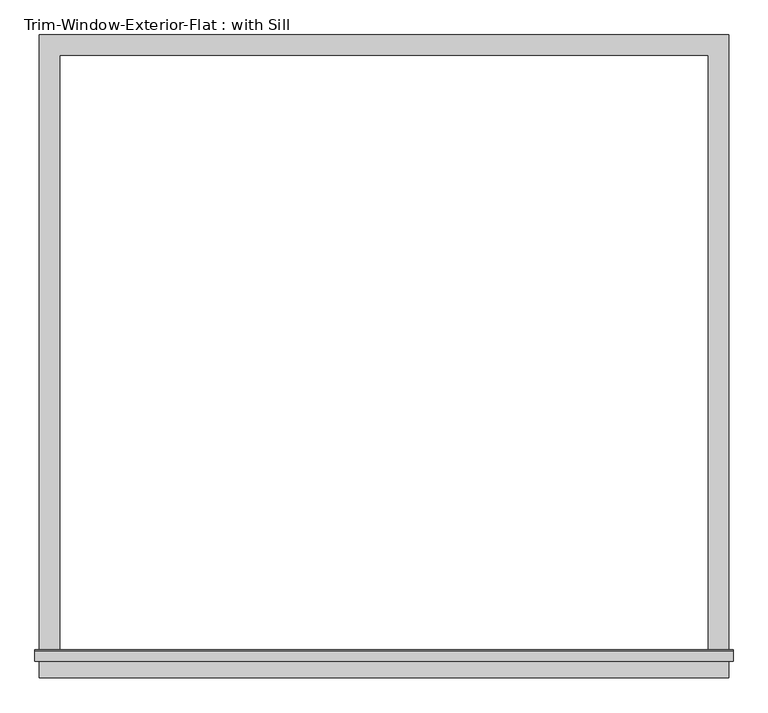
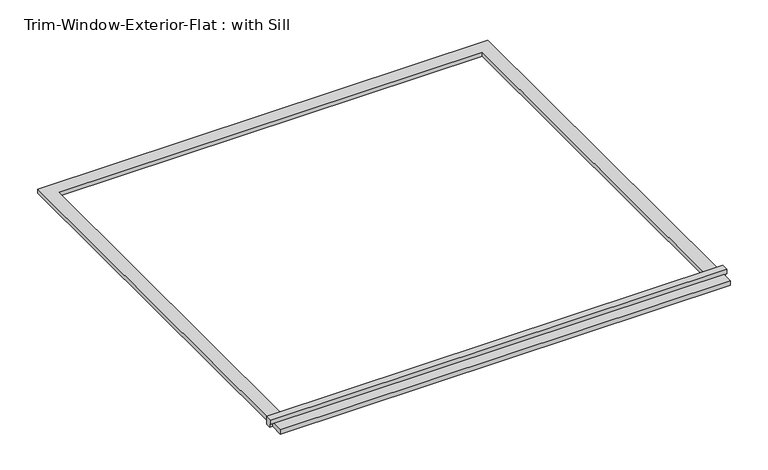
"""IFC4 building model written with IfcOpenShell, lengths in millimetres: proxy geometry, Trim-Window-Exterior-Flat : with Sill."""

from ifc_helpers import new_model, si_unit, frame, origin, origin_with_axes, place, context, project, spatial, polyline, outline, extrude, source, transform, mapped, element, save


def trim_window_exterior_flat_with_sill_c98b2dec(model_context):
    return source(origin(), model_context, "Body", "SweptSolid", [
        extrude(outline(polyline([(971.55, -1698.5823709), (971.55, -1755.7323709), (-971.55, -1755.7323709), (-971.55, -1698.5823709), (971.55, -1698.5823709)])), origin_with_axes(), (0.0, 0.0, 1.0), 19.05),
        extrude(outline(polyline([(-1708.15, 38.1), (-1678.8580645, 38.1), (-1676.4, 19.05), (-1676.4, 0.0), (-1698.5823709, 0.0), (-1698.5823709, 19.05), (-1708.15, 19.05), (-1708.15, 38.1)])), frame((-984.25, 0.0, 0.0), z_axis=(1.0, 0.0, 0.0), x_axis=(0.0, 1.0, 0.0)), (0.0, 0.0, 1.0), 1968.5),
        extrude(outline(polyline([(-971.55, 57.15), (971.55, 57.15), (971.55, -1676.4), (914.4, -1676.4), (914.4, 0.0), (-914.4, 0.0), (-914.4, -1676.4), (-971.55, -1676.4), (-971.55, 57.15)])), origin_with_axes(), (0.0, 0.0, 1.0), 19.05),
    ])


if __name__ == "__main__":
    model = new_model("IFC4")
    model_context = context("Model", 3, world=origin())
    ifc_project = project(units=[si_unit("LENGTHUNIT", "METRE", prefix="MILLI")], contexts=[model_context])
    site = spatial("IfcSite", under=ifc_project)
    building = spatial("IfcBuilding", under=site)
    placement = place(None, origin())
    trim_window_exterior_flat_with_sill_shape = trim_window_exterior_flat_with_sill_c98b2dec(model_context)
    element("IfcBuildingElementProxy", 1, Name="Trim-Window-Exterior-Flat : with Sill", ObjectType="Trim-Window-Exterior-Flat : with Sill", at=placement, inside=building, context=model_context, shape_type="MappedRepresentation", body=[
        mapped(trim_window_exterior_flat_with_sill_shape, transform((0.0, 0.0, 0.0), x_axis=(1.0, 0.0, 0.0), y_axis=(0.0, 1.0, 0.0), z_axis=(0.0, 0.0, 1.0))),
    ])
    save(model, "model.ifc")

# Revit data of these elements
# Type "Trim-Window-Exterior-Flat : with Sill"
#   Trim Width = 0' - 2 1/4"
#   Trim Thickness_Picture Frame = 0' - 1 1/4"
#   Trim Thickness_with Sill = 0' - 0 3/4"
#   Sill Thickness = 0' - 1 1/4"
#   Opening Width [instance default] = 2' - 0"
#   Opening Height [instance default] = 3' - 0"
#   Default Elevation = 4' - 0"
#   Sill = yes
#   Picture Frame = no
#   Trim Material [instance default] = none
# Element 1 (IfcBuildingElementProxy, "Trim-Window-Exterior-Flat : with Sill")
#   Opening Width = 6' - 0"
#   Opening Height = 5' - 6"
#   Trim Material = Clad - White
#   Materials on its faces: "Clad - White"
# Materials
#   "Clad - White": class "Wood", colour RGB 242 242 238, transparency 0, Cost = 0
